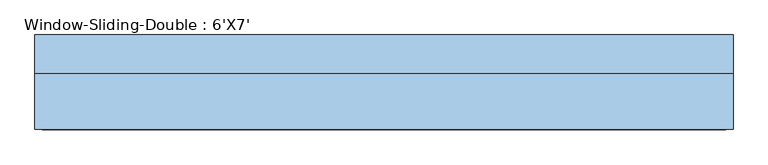
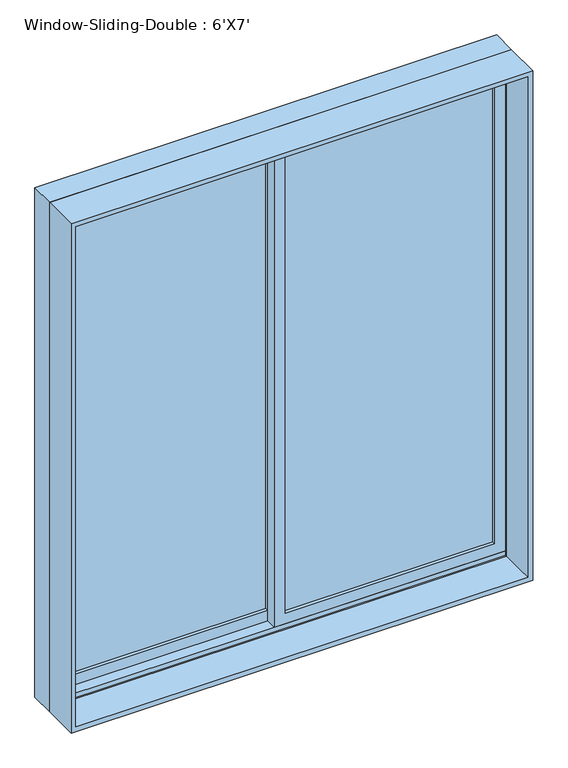
"""IFC4 building model written with IfcOpenShell, lengths in millimetres: window geometry, Window-Sliding-Double : 6'X7'."""

from ifc_helpers import new_model, si_unit, frame, origin, place, context, project, spatial, polyline, outline, extrude, faceted_brep, source, transform, mapped, element, save


def window_sliding_double_6_x7_726fea71(model_context):
    return source(origin(), model_context, "Body", "SolidModel", [
        extrude(outline(polyline([(952.5, 895.35), (3028.95, 895.35), (3028.95, -22.225), (952.5, -22.225), (952.5, 895.35)]), holes=[polyline([(996.95, 22.225), (2984.5, 22.225), (2984.5, 850.9), (996.95, 850.9), (996.95, 22.225)])]), frame((0.0, 34.29, 0.0), z_axis=(0.0, 1.0, 0.0), x_axis=(0.0, 0.0, 1.0)), (0.0, 0.0, 1.0), 44.45),
        extrude(outline(polyline([(933.45, -895.35), (933.45, 22.225), (3028.95, 22.225), (3028.95, -895.35), (933.45, -895.35)]), holes=[polyline([(2984.5, -22.225), (996.95, -22.225), (996.95, -850.9), (2984.5, -850.9), (2984.5, -22.225)])]), frame((0.0, 78.74, 0.0), z_axis=(0.0, 1.0, 0.0), x_axis=(0.0, 0.0, 1.0)), (0.0, 0.0, 1.0), 44.45),
        extrude(outline(polyline([(-22.225, 110.49), (-22.225, 104.14), (-850.9, 104.14), (-850.9, 110.49), (-22.225, 110.49)])), frame((0.0, 0.0, 996.95), z_axis=(0.0, 0.0, 1.0), x_axis=(1.0, 0.0, 0.0)), (0.0, 0.0, 1.0), 1987.55),
        extrude(outline(polyline([(-22.225, 97.79), (-22.225, 91.44), (-850.9, 91.44), (-850.9, 97.79), (-22.225, 97.79)])), frame((0.0, 0.0, 996.95), z_axis=(0.0, 0.0, 1.0), x_axis=(1.0, 0.0, 0.0)), (0.0, 0.0, 1.0), 1987.55),
        extrude(outline(polyline([(850.9, 66.04), (850.9, 59.69), (22.225, 59.69), (22.225, 66.04), (850.9, 66.04)])), frame((0.0, 0.0, 996.95), z_axis=(0.0, 0.0, 1.0), x_axis=(1.0, 0.0, 0.0)), (0.0, 0.0, 1.0), 1987.55),
        extrude(outline(polyline([(850.9, 53.34), (850.9, 46.99), (22.225, 46.99), (22.225, 53.34), (850.9, 53.34)])), frame((0.0, 0.0, 996.95), z_axis=(0.0, 0.0, 1.0), x_axis=(1.0, 0.0, 0.0)), (0.0, 0.0, 1.0), 1987.55),
        extrude(outline(polyline([(3048.0, -914.4), (914.4, -914.4), (914.4, 914.4), (3048.0, 914.4), (3048.0, -914.4)]), holes=[polyline([(3028.95, 895.35), (933.45, 895.35), (933.45, -895.35), (3028.95, -895.35), (3028.95, 895.35)])]), frame((0.0, -118.11, 0.0), z_axis=(0.0, 1.0, 0.0), x_axis=(0.0, 0.0, 1.0)), (0.0, 0.0, 1.0), 146.05),
        faceted_brep([(-914.4, 27.94, 914.4), (-914.4, 129.54, 914.4), (914.4, 129.54, 914.4), (914.4, 27.94, 914.4), (-873.4778905, 129.54, 3007.0778905), (-873.4778905, 123.19, 3007.0778905), (-873.4778905, 123.19, 933.45), (-873.4778905, 129.54, 933.45), (873.4778905, 123.19, 3007.0778905), (873.4778905, 123.19, 933.45), (895.35, 123.19, 933.45), (895.35, 123.19, 3028.95), (-895.35, 123.19, 3028.95), (-895.35, 123.19, 933.45), (-895.35, 27.94, 3028.95), (-895.35, 27.94, 933.45), (-895.35, 34.29, 933.45), (-895.35, 34.29, 952.5), (-895.35, 78.74, 952.5), (-895.35, 78.74, 933.45), (914.4, 27.94, 3048.0), (-914.4, 27.94, 3048.0), (895.35, 27.94, 3028.95), (895.35, 27.94, 933.45), (-914.4, 129.54, 3048.0), (914.4, 129.54, 3048.0), (873.4778905, 129.54, 933.45), (873.4778905, 129.54, 3007.0778905), (895.35, 78.74, 933.45), (895.35, 78.74, 952.5), (895.35, 34.29, 952.5), (895.35, 34.29, 933.45)], [[[0, 1, 2, 3]], [[4, 5, 6, 7]], [[5, 8, 9, 10, 11, 12, 13, 6]], [[12, 14, 15, 16, 17, 18, 19, 13]], [[0, 3, 20, 21], [22, 23, 15, 14]], [[24, 1, 0, 21]], [[2, 1, 24, 25], [4, 7, 26, 27]], [[5, 4, 27, 8]], [[12, 11, 22, 14]], [[21, 20, 25, 24]], [[8, 27, 26, 9]], [[22, 11, 10, 28, 29, 30, 31, 23]], [[20, 3, 2, 25]], [[26, 7, 6, 13, 19, 28, 10, 9]], [[28, 19, 18, 29]], [[29, 18, 17, 30]], [[30, 17, 16, 31]], [[15, 23, 31, 16]]]),
    ])


if __name__ == "__main__":
    model = new_model("IFC4")
    model_context = context("Model", 3, world=origin())
    ifc_project = project(units=[si_unit("LENGTHUNIT", "METRE", prefix="MILLI")], contexts=[model_context])
    site = spatial("IfcSite", under=ifc_project)
    building = spatial("IfcBuilding", under=site)
    placement = place(None, origin())
    window_sliding_double_6_x7_shape = window_sliding_double_6_x7_726fea71(model_context)
    element("IfcWindow", 1, ObjectType="Window-Sliding-Double : 6'X7'", at=placement, inside=building, context=model_context, shape_type="MappedRepresentation", body=[
        mapped(window_sliding_double_6_x7_shape, transform((0.0, 0.0, 0.0), x_axis=(1.0, 0.0, 0.0), y_axis=(0.0, 1.0, 0.0), z_axis=(0.0, 0.0, 1.0))),
    ])
    save(model, "model.ifc")

# Revit data of these elements
# Type "Window-Sliding-Double : 6'X7'"
#   Type Mark = "19"
#   Fire Rating = "0.5h"
#   Assembly Code = "B2020100"
#   Analytic Construction = "Double glazing - domestic"
#   Window Inset [instance default] = 0' - 0"
#   Wall Thickness [instance default] = 0' - 6"
#   Visual Light Transmittance = 0.81
#   Thermal Resistance (R) = 1.8146 (h·ft²·°F)/BTU
#   Solar Heat Gain Coefficient = 0.76
#   Muntin Width = 2' - 8 5/8"
#   Muntin Height = 6' - 6 1/4"
#   Interior Wall Closure [instance default] = 0' - 2 3/4"
#   Heat Transfer Coefficient (U) = 0.5511 BTU/(h·ft²·°F)
#   Frame Extension [instance default] = 0' - 0 1/4"
#   Exterior Wall Closure [instance default] = 0' - 1 1/4"
#   Rough Width = 6' - 0 1/2"
#   Rough Height = 7' - 0 1/2"
#   Height = 7' - 0"
#   Extension Jamb [instance default] = 0' - 2 3/4"
#   Default Sill Height = 3' - 0"
#   Width = 6' - 0"
#   Interior Trim Visibility [instance default] = yes
#   Indicator Visibility [instance default] = yes
#   Exterior Trim Visibility [instance default] = yes
#   Muntin Visibility = yes
#   Extension Jamb Visibility [instance default] = yes
#   Muntin Pattern = Muntin Pattern_2x2 : Muntin Pattern_2x2
#   Interior Trim Material = Wood - Stained
#   Interior Trim = Trim-Window-Interior-Flat : Picture Frame
#   Interior Frame Material = Wood - Stained
#   Glass Panel Material = Glass
#   Exterior Trim Material = Clad - White
#   Exterior Trim = Trim-Window-Exterior-Flat : with Sill
#   Exterior Frame Material = Clad - White
#   Wall Closure = (empty or 0)
# Element 1 (IfcWindow, "Window-Sliding-Double : 6'X7'")
#   Wall Thickness = 0' - 9"
#   Extension Jamb = 0' - 5 3/4"
#   Materials on its faces: "Wood - Stained", "Glass", "Clad - White"
# Materials
#   "Wood - Stained": class "Wood", colour RGB 224 178 126, transparency 0, Cost = 0
#   "Glass": class "Glass", colour RGB 0 128 192, transparency 0.75, Description = "Soda Lime Glass", Cost = 0
#   "Clad - White": class "Wood", colour RGB 242 242 238, transparency 0, Cost = 0
